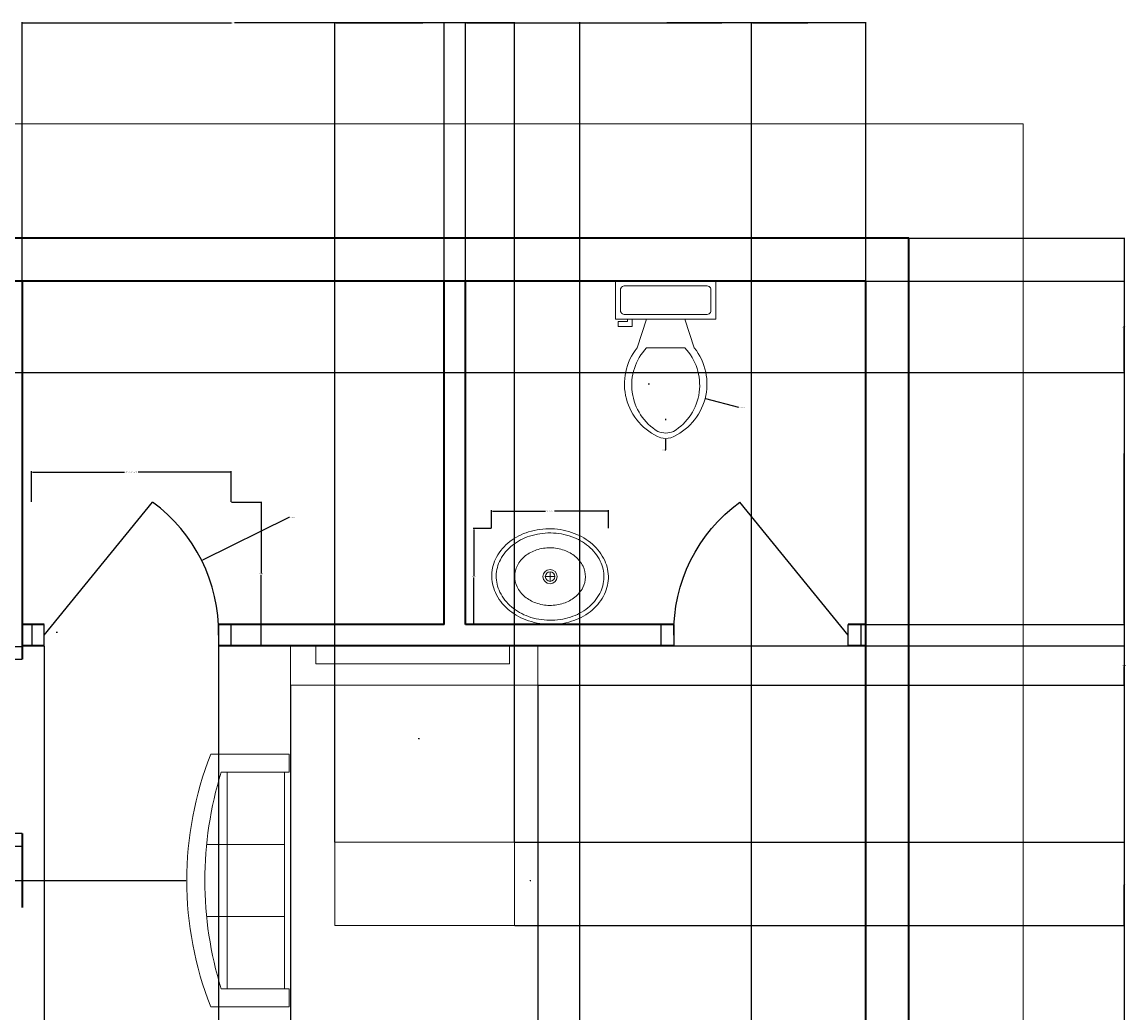
# Model space of a CAD drawing. Units: inches. Extents: x 109 to 572, y -157 to 568.
# Tile 5 of 5: x 341 to 572, y 360 to 568. Entities that reach past the tile are written whole.
import ezdxf

# ---------------------------------------------------------------- set-up
doc = ezdxf.new("R2010")
doc.units = ezdxf.units.IN
for name, color, linetype, lineweight in [('A-ANNO-DIMS', 2, 'Continuous', 18), ('A-FLOR-FIXT', 4, 'Continuous', 18), ('A-WALL', 7, 'Continuous', 35), ('C-PROP', 8, 'Continuous', 18), ('DOOR.', 240, 'Continuous', 25), ('FURNUTURE', 50, 'Continuous', 18)]:
    doc.layers.add(name, color=color, linetype=linetype, lineweight=lineweight)
doc.styles.get("Standard").update_dxf_attribs({"font": 'arial.ttf'})
doc.dimstyles.get("Standard").update_dxf_attribs({"dimtxt": 0.18, "dimasz": 0.18, "dimexe": 0.18, "dimexo": 0.0625, "dimgap": 0.09, "dimtad": 0, "dimtih": 1, "dimtoh": 1, "dimdec": 4, "dimzin": 0, "dimdsep": 46, "dimtxsty": 'Standard', "dimcen": 0.09, "dimadec": 0, "dimazin": 0, "dimtfac": 1, "dimtdec": 4, "dimtofl": 0, "dimtmove": 0, "dimatfit": 3, "dimfxl": 1, "dimtolj": 1, "dimtzin": 0, "dimarcsym": 0})

# ---------------------------------------------------------------- blocks, each defined once
blk = doc.blocks.new('Toilet - top')
for p, q in [((9.5, -6), (9.5, -2)), ((-10, -8.5), (-8, -8.5)), ((-10, -9.5), (-10, -8.5)), ((-8, -8.5), (-8, -8)), ((-7, -8), (-7, -9.5)), ((-4, -8), (-6, -14)), ((4, -8), (6, -14)), ((-7, -9.5), (-10, -9.5)), ((4, -14), (-4, -14))]:
    blk.add_line(p, q)
blk.add_lwpolyline([(10.5, -8), (10.5, 0), (-10.5, 0), (-10.5, -8)], close=True)
for points in [[(-9.5, -2), (-9.5, -6)], [(8.5, -1), (-8.5, -1)], [(-8.5, -7), (8.5, -7)]]:
    blk.add_lwpolyline(points)
for centre, radius, start, end in [((-8.62, -1.88), 0.884, 81.8699, 188.1301), ((8.62, -1.88), 0.884, 351.8699, 98.1301), ((-8.62, -6.12), 0.884, 171.8699, 278.1301), ((8.62, -6.12), 0.884, 261.8699, 8.1301), ((3.52, -21.58), 12.17, 141.4691, 247.9714), ((4.2, -21.82), 11.33, 136.3677, 238.9468), ((-3.52, -21.58), 12.17, 292.0284, 38.5307), ((-4.2, -21.82), 11.33, 301.053, 43.6321), ((0, -27.88), 4, 245.7318, 294.2682), ((0, -29), 4, 254.8605, 285.1395)]:
    blk.add_arc(centre, radius, start, end)
blk = doc.blocks.new('Sofa - Roundback 7 ft.')
for p, q in [((-12.00002, -32.4421), (-12.00003, -6.5971)), ((11.99997, -32.4421), (11.99998, -6.5971)), ((-36.000027, -34), (-36.000027, -11.4696)), ((-35.999844, -13.3819), (35.9998, -13.3819)), ((35.99998, -34), (35.99998, -11.4696)), ((-36.000027, -32.4421), (35.99998, -32.4421))]:
    blk.add_line(p, q)
for points in [[(-36.000027, -34), (-42.000027, -34), (-42.000027, -8)], [(41.99998, -8), (41.99998, -34), (35.99998, -34)]]:
    blk.add_lwpolyline(points)
for centre, radius, start, end in [((0, -114.25), 114.25, 68.43141, 111.5686), ((-0.00001, -127.1968), 121.1968, 72.72033, 107.2797)]:
    blk.add_arc(centre, radius, start, end)
blk = doc.blocks.new('Sink - Oval top')
for p, q in [((-1, 0), (1, 0)), ((0, 1), (0, -1))]:
    blk.add_line(p, q)
for points in [[(-12.23, 0.39, 0.117634), (-11.46, -3.36, 0.104469), (-8.88, -6.8, 0.090016), (-5.08, -9.07, 0.08192), (-0.32, -10.02, 0.08192), (4.49, -9.38, 0.090016), (8.42, -7.36, 0.104469), (11.22, -4.09, 0.117634), (12.23, -0.39, 0.117634), (11.46, 3.36, 0.104469), (8.88, 6.8, 0.090016), (5.08, 9.07, 0.08192), (0.32, 10.02, 0.08192), (-4.49, 9.38, 0.090016), (-8.42, 7.36, 0.104469), (-11.22, 4.09, 0.117634)], [(-11.29, 0.16, 0.118622), (-10.52, -3.25, 0.104678), (-8.07, -6.36, 0.089562), (-4.54, -8.37, 0.081185), (-0.13, -9.15, 0.081185), (4.3, -8.49, 0.089562), (7.89, -6.58, 0.104678), (10.42, -3.55, 0.118622), (11.29, -0.16, 0.118622), (10.52, 3.25, 0.104678), (8.07, 6.36, 0.089562), (4.54, 8.37, 0.081185), (0.13, 9.15, 0.081185), (-4.3, 8.49, 0.089562), (-7.89, 6.58, 0.104678), (-10.42, 3.55, 0.118622)], [(-7.42, 0.08, 0.118283), (-6.91, -2.17, 0.104607), (-5.29, -4.21, 0.089718), (-2.97, -5.53, 0.081436), (-0.07, -6.04, 0.081436), (2.84, -5.59, 0.089718), (5.2, -4.33, 0.104607), (6.86, -2.32, 0.118283), (7.42, -0.08, 0.118283), (6.91, 2.17, 0.104607), (5.29, 4.21, 0.089718), (2.97, 5.53, 0.081436), (0.07, 6.04, 0.081436), (-2.84, 5.59, 0.089718), (-5.2, 4.33, 0.104607), (-6.86, 2.32, 0.118283)]]:
    blk.add_lwpolyline(points, format="xyb", close=True)
for radius in [1.5, 1]:
    blk.add_circle((0, 0), radius)
blk = doc.blocks.new('DOOR-SINGLE-36IN-JAMB')
blk.add_line((0, 0), (-27.91, 22.73))
for points in [[(-2.25, 36.57), (2.25, 36.57), (2.25, 39.21), (-2.25, 39.21)], [(-2.25, -2.64), (2.25, -2.64), (2.25, 0), (-2.25, 0)]]:
    blk.add_lwpolyline(points, close=True)
blk.add_arc((-0.58, 2.67), 33.9, 89.0125, 143.7179)
blk = doc.blocks.new('*D15')
at = {"layer": 'A-ANNO-DIMS', "color": 0, "lineweight": -2, "transparency": 16777216}
for p, q in [((342.53, 467.27), (342.53, 473.66)), ((342.71, 473.48), (362.03, 473.48)), ((384.2, 473.48), (364.88, 473.48)), ((384.38, 467.27), (384.38, 473.66))]:
    blk.add_line(p, q, dxfattribs=at)
at = {"layer": 'A-ANNO-DIMS', "color": 0, "transparency": 16777216}
for points in [[(342.71, 473.51), (342.71, 473.45), (342.53, 473.48)], [(384.2, 473.51), (384.2, 473.45), (384.38, 473.48)]]:
    blk.add_solid(points, dxfattribs=at)
at = {"layer": 'Defpoints', "color": 0, "transparency": 16777216}
for p in [(384.38, 473.48), (342.53, 467.2), (384.38, 467.2)]:
    blk.add_point(p, dxfattribs=at)
at = {"layer": 'A-ANNO-DIMS', "color": 0, "transparency": 16777216, "insert": (363.46, 473.48), "char_height": 0.18, "attachment_point": 5}
blk.add_mtext('\\A1;DOOR & JAMB 42 TYP.', dxfattribs=at)
blk = doc.blocks.new('*D16')
at = {"layer": 'A-ANNO-DIMS', "color": 0, "lineweight": -2, "transparency": 16777216}
for p, q in [((384.44, 467.2), (390.84, 467.2)), ((390.66, 467.02), (390.66, 452.3)), ((390.66, 437.22), (390.66, 451.94)), ((384.44, 437.04), (390.84, 437.04))]:
    blk.add_line(p, q, dxfattribs=at)
at = {"layer": 'A-ANNO-DIMS', "color": 0, "transparency": 16777216}
for points in [[(390.63, 467.02), (390.69, 467.02), (390.66, 467.2)], [(390.63, 437.22), (390.69, 437.22), (390.66, 437.04)]]:
    blk.add_solid(points, dxfattribs=at)
at = {"layer": 'Defpoints', "color": 0, "transparency": 16777216}
for p in [(384.38, 467.2), (384.38, 437.04), (390.66, 437.04)]:
    blk.add_point(p, dxfattribs=at)
at = {"layer": 'A-ANNO-DIMS', "color": 0, "transparency": 16777216, "insert": (390.66, 452.12), "char_height": 0.18, "attachment_point": 5}
blk.add_mtext('\\A1;30 TYP.', dxfattribs=at)
blk = doc.blocks.new('*D21')
at = {"layer": 'A-ANNO-DIMS', "color": 0, "lineweight": -2, "transparency": 16777216}
for p, q in [((438.99, 461.69), (438.99, 465.49)), ((463.54, 461.69), (463.54, 465.49)), ((439.17, 465.31), (450.32, 465.31)), ((463.36, 465.31), (452.2, 465.31))]:
    blk.add_line(p, q, dxfattribs=at)
at = {"layer": 'A-ANNO-DIMS', "color": 0, "transparency": 16777216}
for points in [[(439.17, 465.34), (439.17, 465.28), (438.99, 465.31)], [(463.36, 465.34), (463.36, 465.28), (463.54, 465.31)]]:
    blk.add_solid(points, dxfattribs=at)
at = {"layer": 'Defpoints', "color": 0, "transparency": 16777216}
for p in [(463.54, 465.31), (438.99, 461.62), (463.54, 461.62)]:
    blk.add_point(p, dxfattribs=at)
at = {"layer": 'A-ANNO-DIMS', "color": 0, "transparency": 16777216, "insert": (451.26, 465.31), "char_height": 0.18, "attachment_point": 5}
blk.add_mtext('\\A1;BASIN 25 TYP.', dxfattribs=at)
blk = doc.blocks.new('*D22')
at = {"layer": 'A-ANNO-DIMS', "color": 0, "lineweight": -2, "transparency": 16777216}
for p, q in [((438.92, 461.62), (435.12, 461.62)), ((435.3, 461.44), (435.3, 451.74)), ((435.3, 441.67), (435.3, 451.37)), ((438.92, 441.49), (435.12, 441.49))]:
    blk.add_line(p, q, dxfattribs=at)
at = {"layer": 'A-ANNO-DIMS', "color": 0, "transparency": 16777216}
for points in [[(435.27, 461.44), (435.33, 461.44), (435.3, 461.62)], [(435.27, 441.67), (435.33, 441.67), (435.3, 441.49)]]:
    blk.add_solid(points, dxfattribs=at)
at = {"layer": 'Defpoints', "color": 0, "transparency": 16777216}
for p in [(435.3, 461.62), (438.99, 461.62), (438.99, 441.49)]:
    blk.add_point(p, dxfattribs=at)
at = {"layer": 'A-ANNO-DIMS', "color": 0, "transparency": 16777216, "insert": (435.3, 451.56), "char_height": 0.18, "attachment_point": 5}
blk.add_mtext('\\A1;20 TYP.', dxfattribs=at)
blk = doc.blocks.new('*D44')
at = {"layer": 'A-ANNO-DIMS', "color": 0, "lineweight": -2, "transparency": 16777216}
for p, q in [((526.58, 522.54), (571.85, 522.54)), ((571.67, 522.36), (571.67, 354.72)), ((571.67, 186.72), (571.67, 354.36)), ((526.58, 186.54), (571.85, 186.54))]:
    blk.add_line(p, q, dxfattribs=at)
at = {"layer": 'A-ANNO-DIMS', "color": 0, "transparency": 16777216}
for points in [[(571.64, 522.36), (571.7, 522.36), (571.67, 522.54)], [(571.64, 186.72), (571.7, 186.72), (571.67, 186.54)]]:
    blk.add_solid(points, dxfattribs=at)
at = {"layer": 'Defpoints', "color": 0, "transparency": 16777216}
for p in [(526.52, 522.54), (571.67, 522.54), (526.52, 186.54)]:
    blk.add_point(p, dxfattribs=at)
at = {"layer": 'A-ANNO-DIMS', "color": 0, "transparency": 16777216, "insert": (571.67, 354.54), "char_height": 0.18, "attachment_point": 5}
blk.add_mtext('\\A1;336', dxfattribs=at)
blk = doc.blocks.new('*D46')
at = {"layer": 'A-ANNO-DIMS', "color": 0, "lineweight": -2, "transparency": 16777216}
for p, q in [((340.52, 513.6), (340.52, 567.87)), ((340.7, 567.69), (384.44, 567.69)), ((428.84, 567.69), (385.09, 567.69)), ((429.02, 513.6), (429.02, 567.87))]:
    blk.add_line(p, q, dxfattribs=at)
at = {"layer": 'A-ANNO-DIMS', "color": 0, "transparency": 16777216}
for points in [[(340.7, 567.72), (340.7, 567.66), (340.52, 567.69)], [(428.84, 567.72), (428.84, 567.66), (429.02, 567.69)]]:
    blk.add_solid(points, dxfattribs=at)
at = {"layer": 'Defpoints', "color": 0, "transparency": 16777216}
for p in [(429.02, 567.69), (340.52, 513.54), (429.02, 513.54)]:
    blk.add_point(p, dxfattribs=at)
at = {"layer": 'A-ANNO-DIMS', "color": 0, "transparency": 16777216, "insert": (384.77, 567.69), "char_height": 0.18, "attachment_point": 5}
blk.add_mtext('\\A1;88.5', dxfattribs=at)
blk = doc.blocks.new('*D47')
at = {"layer": 'A-ANNO-DIMS', "color": 0, "lineweight": -2, "transparency": 16777216}
for p, q in [((433.52, 513.6), (433.52, 567.87)), ((433.7, 567.69), (475.3, 567.69)), ((517.34, 567.69), (475.74, 567.69)), ((517.52, 513.6), (517.52, 567.87))]:
    blk.add_line(p, q, dxfattribs=at)
at = {"layer": 'A-ANNO-DIMS', "color": 0, "transparency": 16777216}
for points in [[(433.7, 567.72), (433.7, 567.66), (433.52, 567.69)], [(517.34, 567.72), (517.34, 567.66), (517.52, 567.69)]]:
    blk.add_solid(points, dxfattribs=at)
at = {"layer": 'Defpoints', "color": 0, "transparency": 16777216}
for p in [(517.52, 567.69), (433.52, 513.54), (517.52, 513.54)]:
    blk.add_point(p, dxfattribs=at)
at = {"layer": 'A-ANNO-DIMS', "color": 0, "transparency": 16777216, "insert": (475.52, 567.69), "char_height": 0.18, "attachment_point": 5}
blk.add_mtext('\\A1;84', dxfattribs=at)
blk = doc.blocks.new('*D51')
at = {"layer": 'A-ANNO-DIMS', "color": 0, "lineweight": -2, "transparency": 16777216}
for p, q in [((517.58, 513.54), (571.85, 513.54)), ((571.67, 513.36), (571.67, 477.72)), ((571.67, 441.72), (571.67, 477.36)), ((517.58, 441.54), (571.85, 441.54))]:
    blk.add_line(p, q, dxfattribs=at)
at = {"layer": 'A-ANNO-DIMS', "color": 0, "transparency": 16777216}
for points in [[(571.64, 513.36), (571.7, 513.36), (571.67, 513.54)], [(571.64, 441.72), (571.7, 441.72), (571.67, 441.54)]]:
    blk.add_solid(points, dxfattribs=at)
at = {"layer": 'Defpoints', "color": 0, "transparency": 16777216}
for p in [(517.52, 513.54), (571.67, 513.54), (517.52, 441.54)]:
    blk.add_point(p, dxfattribs=at)
at = {"layer": 'A-ANNO-DIMS', "color": 0, "transparency": 16777216, "insert": (571.67, 477.54), "char_height": 0.18, "attachment_point": 5}
blk.add_mtext('\\A1;72', dxfattribs=at)
blk = doc.blocks.new('*D53')
at = {"layer": 'A-ANNO-DIMS', "color": 0, "lineweight": -2, "transparency": 16777216}
for p, q in [((457.52, 320.1), (457.52, 567.87)), ((457.7, 567.69), (487.3, 567.69)), ((517.34, 567.69), (487.74, 567.69)), ((517.52, 320.1), (517.52, 567.87))]:
    blk.add_line(p, q, dxfattribs=at)
at = {"layer": 'A-ANNO-DIMS', "color": 0, "transparency": 16777216}
for points in [[(457.7, 567.72), (457.7, 567.66), (457.52, 567.69)], [(517.34, 567.72), (517.34, 567.66), (517.52, 567.69)]]:
    blk.add_solid(points, dxfattribs=at)
at = {"layer": 'Defpoints', "color": 0, "transparency": 16777216}
for p in [(517.52, 567.69), (457.52, 320.04), (517.52, 320.04)]:
    blk.add_point(p, dxfattribs=at)
at = {"layer": 'A-ANNO-DIMS', "color": 0, "transparency": 16777216, "insert": (487.52, 567.69), "char_height": 0.18, "attachment_point": 5}
blk.add_mtext('\\A1;60', dxfattribs=at)
blk = doc.blocks.new('*D54')
at = {"layer": 'A-ANNO-DIMS', "color": 0, "lineweight": -2, "transparency": 16777216}
for p, q in [((493.52, 299.47), (493.52, 567.87)), ((493.7, 567.69), (505.3, 567.69)), ((517.34, 567.69), (505.74, 567.69)), ((517.52, 299.47), (517.52, 567.87))]:
    blk.add_line(p, q, dxfattribs=at)
at = {"layer": 'A-ANNO-DIMS', "color": 0, "transparency": 16777216}
for points in [[(493.7, 567.72), (493.7, 567.66), (493.52, 567.69)], [(517.34, 567.72), (517.34, 567.66), (517.52, 567.69)]]:
    blk.add_solid(points, dxfattribs=at)
at = {"layer": 'Defpoints', "color": 0, "transparency": 16777216}
for p in [(517.52, 567.69), (493.52, 299.4), (517.52, 299.4)]:
    blk.add_point(p, dxfattribs=at)
at = {"layer": 'A-ANNO-DIMS', "color": 0, "transparency": 16777216, "insert": (505.52, 567.69), "char_height": 0.18, "attachment_point": 5}
blk.add_mtext('\\A1;24', dxfattribs=at)
blk = doc.blocks.new('*D59')
at = {"layer": 'A-ANNO-DIMS', "color": 0, "lineweight": -2, "transparency": 16777216}
for p, q in [((406.12, 395.88), (406.12, 567.87)), ((406.3, 567.69), (424.58, 567.69)), ((443.63, 567.69), (425.36, 567.69)), ((443.81, 395.88), (443.81, 567.87))]:
    blk.add_line(p, q, dxfattribs=at)
at = {"layer": 'A-ANNO-DIMS', "color": 0, "transparency": 16777216}
for points in [[(406.3, 567.72), (406.3, 567.66), (406.12, 567.69)], [(443.63, 567.72), (443.63, 567.66), (443.81, 567.69)]]:
    blk.add_solid(points, dxfattribs=at)
at = {"layer": 'Defpoints', "color": 0, "transparency": 16777216}
for p in [(443.81, 567.69), (406.12, 395.82), (443.81, 395.82)]:
    blk.add_point(p, dxfattribs=at)
at = {"layer": 'A-ANNO-DIMS', "color": 0, "transparency": 16777216, "insert": (424.97, 567.69), "char_height": 0.18, "attachment_point": 5}
blk.add_mtext('\\A1;37.69', dxfattribs=at)
blk = doc.blocks.new('*D60')
at = {"layer": 'A-ANNO-DIMS', "color": 0, "lineweight": -2, "transparency": 16777216}
for p, q in [((443.88, 395.82), (571.85, 395.82)), ((571.67, 395.64), (571.67, 387.27)), ((571.67, 378.54), (571.67, 386.91)), ((443.88, 378.36), (571.85, 378.36))]:
    blk.add_line(p, q, dxfattribs=at)
at = {"layer": 'A-ANNO-DIMS', "color": 0, "transparency": 16777216}
for points in [[(571.64, 395.64), (571.7, 395.64), (571.67, 395.82)], [(571.64, 378.54), (571.7, 378.54), (571.67, 378.36)]]:
    blk.add_solid(points, dxfattribs=at)
at = {"layer": 'Defpoints', "color": 0, "transparency": 16777216}
for p in [(443.81, 395.82), (443.81, 378.36), (571.67, 378.36)]:
    blk.add_point(p, dxfattribs=at)
at = {"layer": 'A-ANNO-DIMS', "color": 0, "transparency": 16777216, "insert": (571.67, 387.09), "char_height": 0.18, "attachment_point": 5}
blk.add_mtext('\\A1;17.46', dxfattribs=at)
blk = doc.blocks.new('*D61')
at = {"layer": 'A-ANNO-DIMS', "color": 0, "lineweight": -2, "transparency": 16777216}
for p, q in [((396.8, 428.71), (396.8, 105.21)), ((448.7, 428.71), (448.7, 105.21)), ((396.98, 105.39), (422.43, 105.39)), ((448.52, 105.39), (423.08, 105.39))]:
    blk.add_line(p, q, dxfattribs=at)
at = {"layer": 'A-ANNO-DIMS', "color": 0, "transparency": 16777216}
for points in [[(396.98, 105.42), (396.98, 105.36), (396.8, 105.39)], [(448.52, 105.42), (448.52, 105.36), (448.7, 105.39)]]:
    blk.add_solid(points, dxfattribs=at)
at = {"layer": 'Defpoints', "color": 0, "transparency": 16777216}
for p in [(396.8, 428.77), (448.7, 428.77), (448.7, 105.39)]:
    blk.add_point(p, dxfattribs=at)
at = {"layer": 'A-ANNO-DIMS', "color": 0, "transparency": 16777216, "insert": (422.75, 105.39), "char_height": 0.18, "attachment_point": 5}
blk.add_mtext('\\A1;51.9', dxfattribs=at)
blk = doc.blocks.new('*D62')
at = {"layer": 'A-ANNO-DIMS', "color": 0, "lineweight": -2, "transparency": 16777216}
for p, q in [((448.76, 437.04), (571.85, 437.04)), ((571.67, 436.86), (571.67, 433.09)), ((571.67, 428.95), (571.67, 432.72)), ((448.76, 428.77), (571.85, 428.77))]:
    blk.add_line(p, q, dxfattribs=at)
at = {"layer": 'A-ANNO-DIMS', "color": 0, "transparency": 16777216}
for points in [[(571.64, 436.86), (571.7, 436.86), (571.67, 437.04)], [(571.64, 428.95), (571.7, 428.95), (571.67, 428.77)]]:
    blk.add_solid(points, dxfattribs=at)
at = {"layer": 'Defpoints', "color": 0, "transparency": 16777216}
for p in [(448.7, 437.04), (571.67, 437.04), (448.7, 428.77)]:
    blk.add_point(p, dxfattribs=at)
at = {"layer": 'A-ANNO-DIMS', "color": 0, "transparency": 16777216, "insert": (571.67, 432.91), "char_height": 0.18, "attachment_point": 5}
blk.add_mtext('\\A1;8.266', dxfattribs=at)
blk = doc.blocks.new('*D66')
at = {"layer": 'A-ANNO-DIMS', "color": 0, "lineweight": -2, "transparency": 16777216}
for p, q in [((457.52, 219.6), (457.52, 567.87)), ((457.7, 567.69), (475.3, 567.69)), ((493.34, 567.69), (475.74, 567.69)), ((493.52, 219.6), (493.52, 567.87))]:
    blk.add_line(p, q, dxfattribs=at)
at = {"layer": 'A-ANNO-DIMS', "color": 0, "transparency": 16777216}
for points in [[(457.7, 567.72), (457.7, 567.66), (457.52, 567.69)], [(493.34, 567.72), (493.34, 567.66), (493.52, 567.69)]]:
    blk.add_solid(points, dxfattribs=at)
at = {"layer": 'Defpoints', "color": 0, "transparency": 16777216}
for p in [(493.52, 567.69), (457.52, 219.54), (493.52, 219.54)]:
    blk.add_point(p, dxfattribs=at)
at = {"layer": 'A-ANNO-DIMS', "color": 0, "transparency": 16777216, "insert": (475.52, 567.69), "char_height": 0.18, "attachment_point": 5}
blk.add_mtext('\\A1;36', dxfattribs=at)
blk = doc.blocks.new('*D68')
at = {"layer": 'A-ANNO-DIMS', "color": 0, "lineweight": -2, "transparency": 16777216}
for p, q in [((216.08, 513.54), (571.85, 513.54)), ((571.67, 513.36), (571.67, 504.14)), ((571.67, 494.56), (571.67, 503.78)), ((216.08, 494.38), (571.85, 494.38))]:
    blk.add_line(p, q, dxfattribs=at)
at = {"layer": 'A-ANNO-DIMS', "color": 0, "transparency": 16777216}
for points in [[(571.64, 513.36), (571.7, 513.36), (571.67, 513.54)], [(571.64, 494.56), (571.7, 494.56), (571.67, 494.38)]]:
    blk.add_solid(points, dxfattribs=at)
at = {"layer": 'Defpoints', "color": 0, "transparency": 16777216}
for p in [(216.02, 513.54), (216.02, 494.38), (571.67, 494.38)]:
    blk.add_point(p, dxfattribs=at)
at = {"layer": 'A-ANNO-DIMS', "color": 0, "transparency": 16777216, "insert": (571.67, 503.96), "char_height": 0.18, "attachment_point": 5}
blk.add_mtext('\\A1;19.164', dxfattribs=at)
blk = doc.blocks.new('*D71')
at = {"layer": 'A-ANNO-DIMS', "color": 0, "lineweight": -2, "transparency": 16777216}
for p, q in [((345.17, 436.98), (345.17, 105.21)), ((381.74, 436.98), (381.74, 105.21)), ((345.35, 105.39), (363.06, 105.39)), ((381.56, 105.39), (363.85, 105.39))]:
    blk.add_line(p, q, dxfattribs=at)
at = {"layer": 'A-ANNO-DIMS', "color": 0, "transparency": 16777216}
for points in [[(345.35, 105.42), (345.35, 105.36), (345.17, 105.39)], [(381.56, 105.42), (381.56, 105.36), (381.74, 105.39)]]:
    blk.add_solid(points, dxfattribs=at)
at = {"layer": 'Defpoints', "color": 0, "transparency": 16777216}
for p in [(345.17, 437.04), (381.74, 437.04), (381.74, 105.39)]:
    blk.add_point(p, dxfattribs=at)
at = {"layer": 'A-ANNO-DIMS', "color": 0, "transparency": 16777216, "insert": (363.46, 105.39), "char_height": 0.18, "attachment_point": 5}
blk.add_mtext('\\A1;36.57', dxfattribs=at)
blk = doc.blocks.new('*D72')
at = {"layer": 'A-ANNO-DIMS', "color": 0, "lineweight": -2, "transparency": 16777216}
for p, q in [((396.45, 463.96), (378.38, 455.01)), ((396.63, 463.96), (396.45, 463.96)), ((347.84, 439.78), (347.84, 439.96)), ((347.75, 439.87), (347.93, 439.87))]:
    blk.add_line(p, q, dxfattribs=at)
at = {"layer": 'A-ANNO-DIMS', "color": 0, "transparency": 16777216}
blk.add_solid([(378.37, 455.04), (378.4, 454.98), (378.22, 454.93)], dxfattribs=at)
at = {"layer": 'Defpoints', "color": 0, "transparency": 16777216}
for p in [(378.22, 454.93), (347.84, 439.87)]:
    blk.add_point(p, dxfattribs=at)
at = {"layer": 'A-ANNO-DIMS', "color": 0, "transparency": 16777216, "insert": (397.23, 463.96), "char_height": 0.18, "attachment_point": 5}
blk.add_mtext('\\A1;5X R33.9', dxfattribs=at)
blk = doc.blocks.new('*D73')
at = {"layer": 'A-ANNO-DIMS', "color": 0, "lineweight": -2, "transparency": 16777216}
for p, q in [((423.67, 417.59), (423.85, 417.59)), ((423.76, 417.5), (423.76, 417.68)), ((423.77, 295.21), (423.77, 340.92)), ((423.95, 295.21), (423.77, 295.21))]:
    blk.add_line(p, q, dxfattribs=at)
at = {"layer": 'A-ANNO-DIMS', "color": 0, "transparency": 16777216}
blk.add_solid([(423.8, 340.92), (423.74, 340.92), (423.77, 341.1)], dxfattribs=at)
at = {"layer": 'Defpoints', "color": 0, "transparency": 16777216}
for p in [(423.76, 417.59), (423.77, 341.1)]:
    blk.add_point(p, dxfattribs=at)
at = {"layer": 'A-ANNO-DIMS', "color": 0, "transparency": 16777216, "insert": (424.62, 295.21), "char_height": 0.18, "attachment_point": 5}
blk.add_mtext('\\A1;2X R76.49', dxfattribs=at)
blk = doc.blocks.new('*D74')
at = {"layer": 'A-ANNO-DIMS', "color": 0, "lineweight": -2, "transparency": 16777216}
for p, q in [((331.8, 387.8), (374.88, 387.8)), ((447.07, 387.8), (447.25, 387.8)), ((447.16, 387.71), (447.16, 387.89))]:
    blk.add_line(p, q, dxfattribs=at)
at = {"layer": 'A-ANNO-DIMS', "color": 0, "transparency": 16777216}
blk.add_solid([(374.88, 387.83), (374.88, 387.77), (375.06, 387.8)], dxfattribs=at)
at = {"layer": 'Defpoints', "color": 0, "transparency": 16777216}
for p in [(375.06, 387.8), (447.16, 387.8)]:
    blk.add_point(p, dxfattribs=at)
at = {"layer": 'A-ANNO-DIMS', "color": 0, "transparency": 16777216, "insert": (331.21, 387.8), "char_height": 0.18, "attachment_point": 5}
blk.add_mtext('\\A1;2X R72.1', dxfattribs=at)
blk = doc.blocks.new('*D75')
at = {"layer": 'A-ANNO-DIMS', "color": 0, "lineweight": -2, "transparency": 16777216}
for p, q in [((471.91, 491.96), (472.09, 491.96)), ((472, 491.87), (472, 492.05)), ((490.83, 487.01), (483.94, 488.82))]:
    blk.add_line(p, q, dxfattribs=at)
at = {"layer": 'A-ANNO-DIMS', "color": 0, "transparency": 16777216}
blk.add_solid([(483.95, 488.85), (483.93, 488.79), (483.77, 488.87)], dxfattribs=at)
at = {"layer": 'Defpoints', "color": 0, "transparency": 16777216}
for p in [(472, 491.96), (483.77, 488.87)]:
    blk.add_point(p, dxfattribs=at)
at = {"layer": 'A-ANNO-DIMS', "color": 0, "transparency": 16777216, "insert": (491.5, 487.01), "char_height": 0.18, "attachment_point": 5}
blk.add_mtext('\\A1;4X R12.17', dxfattribs=at)
blk = doc.blocks.new('*D77')
at = {"layer": 'A-ANNO-DIMS', "color": 0, "lineweight": -2, "transparency": 16777216}
for p, q in [((475.43, 484.54), (475.61, 484.54)), ((475.52, 484.45), (475.52, 484.63)), ((475.52, 478.14), (475.52, 480.36)), ((475.34, 478.14), (475.52, 478.14))]:
    blk.add_line(p, q, dxfattribs=at)
at = {"layer": 'A-ANNO-DIMS', "color": 0, "transparency": 16777216}
blk.add_solid([(475.49, 480.36), (475.55, 480.36), (475.52, 480.54)], dxfattribs=at)
at = {"layer": 'Defpoints', "color": 0, "transparency": 16777216}
for p in [(475.52, 484.54), (475.52, 480.54)]:
    blk.add_point(p, dxfattribs=at)
at = {"layer": 'A-ANNO-DIMS', "color": 0, "transparency": 16777216, "insert": (474.9, 478.14), "char_height": 0.18, "attachment_point": 5}
blk.add_mtext('\\A1;4X R4', dxfattribs=at)

msp = doc.modelspace()

# ---------------------------------------------------------------- linework, layer by layer
at = {"layer": 'A-WALL'}
for p, q in [((526.5195, 522.5398), (211.5195, 522.5398)), ((526.5195, 186.5398), (526.5195, 522.5398)), ((517.5195, 513.5398), (211.5195, 513.5398)), ((340.5195, 513.5398), (340.5195, 434.2056)), ((429.0195, 441.5398), (429.0195, 513.5398)), ((433.5195, 441.5398), (433.5195, 513.5398)), ((517.5195, 195.5398), (517.5195, 513.5398)), ((345.1719, 441.5398), (340.5195, 441.5398)), ((429.0195, 441.5398), (381.7057, 441.5398)), ((477.257, 441.5398), (433.5195, 441.5398)), ((517.5195, 441.5398), (513.7908, 441.5398)), ((345.1719, 437.0398), (340.5195, 437.0398)), ((477.221, 437.0398), (381.7416, 437.0398)), ((517.5195, 437.0398), (513.7908, 437.0398)), ((340.5195, 397.6358), (340.5195, 382.1753))]:
    msp.add_line(p, q, dxfattribs=at)
at = {"layer": 'C-PROP'}
for p, q in [((550.5195, 546.5398), (130.5195, 546.5398)), ((550.5195, 126.5398), (550.5195, 546.5398))]:
    msp.add_line(p, q, dxfattribs=at)
at = {"layer": 'FURNUTURE'}
for points in [[(396.8044, 437.0398), (448.7025, 437.0398), (448.7025, 428.7734), (396.8044, 428.7734)], [(402.1437, 437.0398), (442.7224, 437.0398), (442.7224, 433.2615), (402.1437, 433.2615)], [(406.1243, 378.3567), (443.8138, 378.3567), (443.8138, 395.8173), (406.1243, 395.8173)]]:
    msp.add_lwpolyline(points, close=True, dxfattribs=at)

# ---------------------------------------------------------------- block references
at = {"layer": 'A-FLOR-FIXT'}
for name, p in [('Toilet - top', (475.5161, 513.5398)), ('Sink - Oval top', (451.2607, 451.5556))]:
    msp.add_blockref(name, p, dxfattribs=at)
at = {"layer": 'DOOR.', "rotation": 269.9999999999994}
msp.add_blockref('DOOR-SINGLE-36IN-JAMB', (345.1719, 439.2898), dxfattribs=at)
at = {"layer": 'DOOR.', "extrusion": (0, 0, -1), "zscale": -1, "rotation": 269.9999999999995}
msp.add_blockref('DOOR-SINGLE-36IN-JAMB', (-513.7908, 439.2898), dxfattribs=at)
at = {"layer": 'DOOR.'}
msp.add_blockref('DOOR-SINGLE-36IN-JAMB', (338.2695, 397.6358), dxfattribs=at)
at = {"layer": 'FURNUTURE', "xscale": 0.6311149755578328, "yscale": 0.6311149755578328, "zscale": 0.6311149755578328, "rotation": 89.99999999999825}
msp.add_blockref('Sofa - Roundback 7 ft.', (375.058, 387.7979), dxfattribs=at)

# ---------------------------------------------------------------- dimensions: what is measured, and where the dimension line sits
at = {"layer": 'A-ANNO-DIMS'}
for base, p1, p2, override, picture, middle in [((429.0195, 567.6898), (340.5195, 513.5398), (429.0195, 513.5398), {"dimdec": 1, "dimlfac": 1, "dimrnd": 0, "dimzin": 0, "dimdsep": 46, "dimlunit": 2}, '*D46', (384.7695, 567.6898)), ((443.8138, 567.6898), (406.1243, 395.8173), (443.8138, 395.8173), {"dimdec": 2, "dimlfac": 1, "dimrnd": 0, "dimzin": 0, "dimdsep": 46, "dimlunit": 2}, '*D59', (424.9691, 567.6898)), ((517.5195, 567.6898), (433.5195, 513.5398), (517.5195, 513.5398), {"dimdec": 0, "dimlfac": 1, "dimrnd": 0, "dimzin": 0, "dimdsep": 46, "dimlunit": 2}, '*D47', (475.5195, 567.6898)), ((517.5195, 567.6898), (457.5195, 320.0398), (517.5195, 320.0398), {"dimdec": 0, "dimlfac": 1, "dimrnd": 0, "dimzin": 0, "dimdsep": 46, "dimlunit": 2}, '*D53', (487.5195, 567.6898)), ((493.5195, 567.6898), (457.5195, 219.5398), (493.5195, 219.5398), {"dimdec": 0, "dimlfac": 1, "dimrnd": 0, "dimzin": 0, "dimdsep": 46, "dimlunit": 2}, '*D66', (475.5195, 567.6898)), ((517.5195, 567.6898), (493.5195, 299.4036), (517.5195, 299.4036), {"dimdec": 0, "dimlfac": 1, "dimrnd": 0, "dimzin": 0, "dimdsep": 46, "dimlunit": 2}, '*D54', (505.5195, 567.6898)), ((381.7416, 105.3898), (345.1719, 437.0398), (381.7416, 437.0398), {"dimdec": 2, "dimlfac": 1, "dimrnd": 0, "dimzin": 0, "dimdsep": 46, "dimlunit": 2}, '*D71', (363.4567, 105.3898)), ((448.7025, 105.3898), (396.8044, 428.7734), (448.7025, 428.7734), {"dimdec": 1, "dimlfac": 1, "dimrnd": 0, "dimzin": 0, "dimdsep": 46, "dimlunit": 2}, '*D61', (422.7534, 105.3898))]:
    dim = msp.add_linear_dim(base=base, p1=p1, p2=p2, dimstyle='Standard', override=override, dxfattribs=at)
    dim.commit()
    dim.dimension.update_dxf_attribs({"geometry": picture, "text_midpoint": middle})
for base, p1, p2, override, picture, middle in [((571.6695, 522.5398), (526.5195, 186.5398), (526.5195, 522.5398), {"dimdec": 0, "dimlfac": 1, "dimrnd": 0, "dimzin": 0, "dimdsep": 46, "dimlunit": 2}, '*D44', (571.6695, 354.5398)), ((571.6695, 494.3755), (216.0195, 513.5398), (216.0195, 494.3755), {"dimdec": 3, "dimlfac": 1, "dimrnd": 0, "dimzin": 0, "dimdsep": 46, "dimlunit": 2}, '*D68', (571.6695, 503.9576)), ((571.6695, 513.5398), (517.5195, 441.5398), (517.5195, 513.5398), {"dimdec": 0, "dimlfac": 1, "dimrnd": 0, "dimzin": 0, "dimdsep": 46, "dimlunit": 2}, '*D51', (571.6695, 477.5398)), ((571.6695, 437.0398), (448.7025, 428.7734), (448.7025, 437.0398), {"dimdec": 3, "dimlfac": 1, "dimrnd": 0, "dimzin": 0, "dimdsep": 46, "dimlunit": 2}, '*D62', (571.6695, 432.9066)), ((571.6695, 378.3567), (443.8138, 395.8173), (443.8138, 378.3567), {"dimdec": 2, "dimlfac": 1, "dimrnd": 0, "dimzin": 0, "dimdsep": 46, "dimlunit": 2}, '*D60', (571.6695, 387.087))]:
    dim = msp.add_linear_dim(base=base, p1=p1, p2=p2, angle=90, dimstyle='Standard', override=override, dxfattribs=at)
    dim.commit()
    dim.dimension.update_dxf_attribs({"geometry": picture, "text_midpoint": middle})
for center, mpoint, text, override, picture, middle in [((471.9966, 491.9593), (483.7662, 488.867), '4X <>', {"dimdec": 2, "dimlfac": 1, "dimrnd": 0, "dimzin": 0, "dimdsep": 46, "dimlunit": 2}, '*D75', (490.8279, 487.0115)), ((475.5161, 484.5398), (475.516, 480.5398), '4X <>', {"dimdec": 0, "dimlfac": 1, "dimrnd": 0, "dimzin": 0, "dimdsep": 46, "dimlunit": 2}, '*D77', (474.9042, 478.1398)), ((347.845, 439.874), (378.2204, 454.9292), '5X <>', {"dimdec": 1, "dimlfac": 1, "dimrnd": 0, "dimzin": 0, "dimdsep": 46, "dimlunit": 2}, '*D72', (397.2291, 463.9623)), ((423.7646, 417.5934), (423.765, 341.1043), '2X <>', {"dimdec": 2, "dimlfac": 1, "dimrnd": 0, "dimzin": 0, "dimdsep": 46, "dimlunit": 2}, '*D73', (424.6202, 295.2108)), ((447.1629, 387.7979), (375.058, 387.798), '2X <>', {"dimdec": 1, "dimlfac": 1, "dimrnd": 0, "dimzin": 0, "dimdsep": 46, "dimlunit": 2}, '*D74', (331.7951, 387.7981))]:
    dim = msp.add_radius_dim(center=center, mpoint=mpoint, text=text, dimstyle='Standard', override=override, dxfattribs=at)
    dim.commit()
    dim.dimension.update_dxf_attribs({"geometry": picture, "text_midpoint": middle, "dimtype": 164})
for base, p1, p2, text, picture, middle in [((384.3807, 473.4798), (342.5328, 467.2026), (384.3807, 467.2026), 'DOOR & JAMB <> TYP.', '*D15', (363.4567, 473.4798)), ((463.5361, 465.3066), (438.9852, 461.6239), (463.5361, 461.6239), 'BASIN <> TYP.', '*D21', (451.2607, 465.3066))]:
    dim = msp.add_linear_dim(base=base, p1=p1, p2=p2, text=text, dimstyle='Standard', override={"dimdec": 0, "dimlfac": 1, "dimrnd": 0, "dimzin": 0, "dimdsep": 46, "dimlunit": 2}, dxfattribs=at)
    dim.commit()
    dim.dimension.update_dxf_attribs({"geometry": picture, "text_midpoint": middle})
for base, p1, p2, angle, picture, middle in [((390.6579, 437.0398), (384.3807, 467.2026), (384.3807, 437.0398), 270, '*D16', (390.6579, 452.1212)), ((435.3026, 461.6239), (438.9852, 441.4873), (438.9852, 461.6239), 90, '*D22', (435.3026, 451.5556))]:
    dim = msp.add_linear_dim(base=base, p1=p1, p2=p2, angle=angle, text='<> TYP.', dimstyle='Standard', override={"dimdec": 0, "dimlfac": 1, "dimrnd": 0, "dimzin": 0, "dimdsep": 46, "dimlunit": 2}, dxfattribs=at)
    dim.commit()
    dim.dimension.update_dxf_attribs({"geometry": picture, "text_midpoint": middle})

doc.saveas('drawing.dxf')
